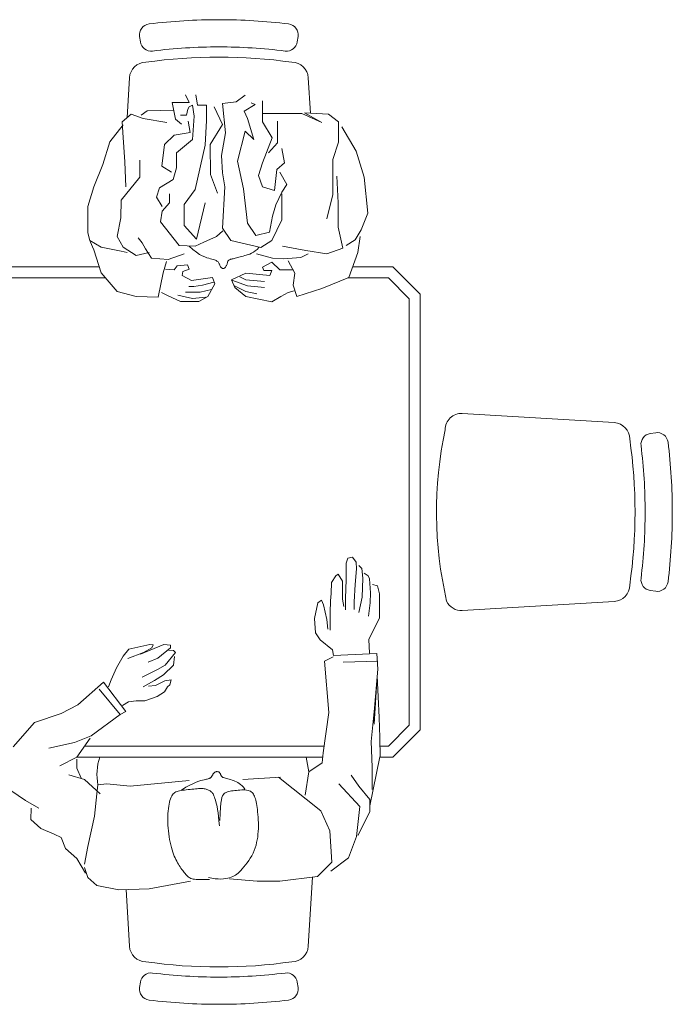
# Model space of a CAD drawing. Units: inches. Extents: x 1913 to 5309, y 1003 to 1733.
# Tile 6 of 23: x 2248 to 2284, y 1415 to 1469. Entities that reach past the tile are written whole.
import ezdxf

# ---------------------------------------------------------------- set-up
doc = ezdxf.new("R2010")
doc.units = ezdxf.units.IN
doc.layers.add('A-FURN', color=8, linetype='Continuous', lineweight=18)

# ---------------------------------------------------------------- blocks, each defined once
blk = doc.blocks.new('A$C421907B3')
for p, q in [((0.3742, 1.1891), (0.3928, 1.2157)), ((0.4726, 1.2115), (0.5176, 1.1724)), ((0.3229, 1.1605), (0.3394, 1.1788)), ((0.3394, 1.1788), (0.36, 1.1787)), ((0.36, 1.1646), (0.3742, 1.1891)), ((0.3126, 1.1359), (0.3229, 1.1605)), ((0.5176, 1.1724), (0.5341, 1.1234)), ((0.4808, 1.0989), (0.4706, 1.1459)), ((0.2861, 1.1152), (0.3066, 1.1235)), ((0.3066, 1.1235), (0.3126, 1.1359)), ((0.4378, 1.1255), (0.454, 1.0947)), ((0.5341, 1.1234), (0.5503, 1.0926)), ((0.2676, 1.0948), (0.2861, 1.1152)), ((0.4132, 1.0806), (0.4212, 1.1093)), ((0.241, 1.0786), (0.2676, 1.0948)), ((0.4335, 1.0947), (0.4152, 1.0865)), ((0.45, 1.0947), (0.4335, 1.0947)), ((0.454, 1.0947), (0.489, 1.0702)), ((0.493, 1.0681), (0.4808, 1.0989)), ((0.5503, 1.0926), (0.5914, 1.0456)), ((0.2328, 1.0745), (0.2183, 1.0579)), ((0.2511, 1.0807), (0.2328, 1.0745)), ((0.2573, 1.0807), (0.2901, 1.0744)), ((0.2901, 1.0744), (0.3454, 1.062)), ((0.3864, 1.0516), (0.4132, 1.0806)), ((0.5322, 1.015), (0.493, 1.0681)), ((1.3858, 1.0635), (1.4011, 1.0699)), ((1.4031, 1.0709), (1.3905, 1.0498)), ((1.4171, 1.0745), (1.4031, 1.0709)), ((1.4656, 1.0745), (1.4171, 1.0745)), ((1.5014, 1.0634), (1.4656, 1.0745)), ((0.2183, 1.0579), (0.2102, 1.0171)), ((0.3454, 1.062), (0.3864, 1.0578)), ((0.3864, 1.0578), (0.4029, 1.0557)), ((0.4029, 1.0557), (0.4049, 1.0395)), ((0.5791, 1.0535), (0.532, 1.0149)), ((1.3094, 1.0205), (1.3433, 1.0498)), ((1.3433, 1.0498), (1.3858, 1.0635)), ((1.3905, 1.0498), (1.3831, 1.0131)), ((1.5426, 1.0469), (1.5014, 1.0634)), ((0.4049, 1.0395), (0.4006, 0.9963)), ((0.538, 1.0045), (0.5914, 1.0456)), ((0.5958, 1.0315), (0.5832, 1.0366)), ((0.618, 1.0218), (0.5958, 1.0315)), ((1.5838, 1.034), (1.5426, 1.0469)), ((1.615, 1.0092), (1.5838, 1.034)), ((0.2102, 1.0171), (0.2122, 0.9615)), ((0.532, 1.0149), (0.538, 1.0045)), ((0.6395, 1.0092), (0.618, 1.0218)), ((1.3001, 0.9856), (1.3094, 1.0205)), ((1.3831, 1.0131), (1.3811, 1.0021)), ((1.3904, 1.0094), (1.4104, 1.0204)), ((1.4104, 1.0204), (1.4443, 1.0139)), ((1.4443, 1.0139), (1.4768, 1.013)), ((1.4768, 1.013), (1.5193, 0.979)), ((0.4006, 0.9963), (0.4108, 0.8878)), ((0.5491, 1.0108), (0.5557, 0.9996)), ((0.5557, 0.9996), (0.5572, 0.9855)), ((0.635, 1.001), (0.6461, 0.9722)), ((0.6521, 0.9988), (0.6395, 1.0092)), ((0.6609, 0.9603), (0.6521, 0.9988)), ((1.3751, 0.9856), (1.3904, 1.0094)), ((1.5014, 1.0047), (1.5472, 1.0065)), ((1.5472, 1.0065), (1.5918, 1.0092)), ((1.5918, 1.0092), (1.621, 1.011)), ((1.621, 1.011), (1.6349, 0.9945)), ((0.5572, 0.9855), (0.5572, 0.9693)), ((0.6609, 0.9344), (0.6432, 0.9774)), ((1.2987, 0.9453), (1.3001, 0.9856)), ((1.3811, 0.9617), (1.3751, 0.9856)), ((1.3984, 0.9745), (1.4077, 0.9819)), ((1.5193, 0.979), (1.5505, 0.979)), ((1.6349, 0.9945), (1.627, 0.9725)), ((0.2122, 0.9615), (0.2264, 0.8858)), ((0.5572, 0.9693), (0.5653, 0.947)), ((0.5832, 0.9729), (0.595, 0.9515)), ((0.5854, 0.9499), (0.5846, 0.9626)), ((0.6009, 0.9744), (0.615, 0.9462)), ((0.6283, 0.9633), (0.6357, 0.9455)), ((0.6461, 0.9722), (0.655, 0.9566)), ((0.6602, 0.9544), (0.6609, 0.9603)), ((1.3705, 0.9571), (1.3877, 0.9681)), ((1.3877, 0.9681), (1.3984, 0.9745)), ((1.627, 0.9725), (1.6196, 0.9294)), ((1.6409, 0.9652), (1.6329, 0.9762)), ((1.6421, 0.9163), (1.6409, 0.9652)), ((0.5653, 0.947), (0.5742, 0.9337)), ((0.5942, 0.933), (0.5854, 0.9499)), ((0.595, 0.9515), (0.6053, 0.9352)), ((0.615, 0.9462), (0.6232, 0.9322)), ((0.6357, 0.9455), (0.655, 0.9225)), ((0.655, 0.9566), (0.6602, 0.9544)), ((1.3432, 0.9361), (1.2987, 0.9453)), ((1.3678, 0.9269), (1.3705, 0.9571)), ((1.3937, 0.9067), (1.4369, 0.9406)), ((1.4369, 0.9406), (1.4568, 0.9378)), ((1.4655, 0.9378), (1.4827, 0.9479)), ((1.4827, 0.9479), (1.4994, 0.9423)), ((1.4994, 0.9423), (1.5146, 0.9176)), ((0.2929, 0.922), (0.2977, 0.923)), ((0.2977, 0.923), (0.3027, 0.924)), ((0.3027, 0.924), (0.3078, 0.9248)), ((0.3078, 0.9248), (0.3131, 0.9255)), ((0.3131, 0.9255), (0.3184, 0.9261)), ((0.3184, 0.9261), (0.3238, 0.9266)), ((0.3238, 0.9266), (0.3293, 0.927)), ((0.3293, 0.927), (0.3347, 0.9272)), ((0.3347, 0.9272), (0.34, 0.9272)), ((0.34, 0.9272), (0.3452, 0.9272)), ((0.3452, 0.9272), (0.3502, 0.927)), ((0.3502, 0.927), (0.355, 0.9267)), ((0.355, 0.9267), (0.3595, 0.9262)), ((0.3595, 0.9262), (0.3638, 0.9257)), ((0.3638, 0.9257), (0.3677, 0.925)), ((0.3677, 0.925), (0.3713, 0.9242)), ((0.3713, 0.9242), (0.3746, 0.9233)), ((0.3746, 0.9233), (0.3776, 0.9223)), ((0.3776, 0.9223), (0.3803, 0.9212)), ((0.5742, 0.9337), (0.5832, 0.9278)), ((0.5832, 0.9278), (0.5869, 0.9233)), ((0.5869, 0.9233), (0.5957, 0.9211)), ((0.5957, 0.9211), (0.5942, 0.933)), ((0.6053, 0.9352), (0.6232, 0.9166)), ((0.6232, 0.9322), (0.6461, 0.9129)), ((0.6498, 0.9166), (0.6506, 0.9263)), ((0.655, 0.9225), (0.6594, 0.9225)), ((0.6594, 0.9225), (0.6609, 0.9344)), ((1.2907, 0.904), (1.3013, 0.9269)), ((1.3013, 0.9269), (1.3073, 0.9388)), ((1.3645, 0.9296), (1.3432, 0.9361)), ((1.3505, 0.9315), (1.3492, 0.9159)), ((1.3784, 0.8975), (1.3678, 0.9269)), ((1.4568, 0.9378), (1.4721, 0.924)), ((1.4721, 0.924), (1.4887, 0.924)), ((1.5286, 0.9203), (1.5392, 0.9386)), ((1.5392, 0.9386), (1.5791, 0.9331)), ((1.5791, 0.9331), (1.5963, 0.9157)), ((0.25, 0.9031), (0.2524, 0.9047)), ((0.2524, 0.9047), (0.2548, 0.9063)), ((0.2548, 0.9063), (0.2573, 0.9078)), ((0.2573, 0.9078), (0.26, 0.9094)), ((0.26, 0.9094), (0.2628, 0.911)), ((0.2628, 0.911), (0.2657, 0.9125)), ((0.2657, 0.9125), (0.2689, 0.914)), ((0.2689, 0.914), (0.2723, 0.9155)), ((0.2723, 0.9155), (0.2759, 0.9169)), ((0.2759, 0.9169), (0.2797, 0.9183)), ((0.2797, 0.9183), (0.2839, 0.9196)), ((0.2839, 0.9196), (0.2883, 0.9208)), ((0.2883, 0.9208), (0.2929, 0.922)), ((0.3803, 0.9212), (0.3826, 0.92)), ((0.3826, 0.92), (0.3847, 0.9187)), ((0.3847, 0.9187), (0.3864, 0.9173)), ((0.3864, 0.9173), (0.3878, 0.9158)), ((0.3878, 0.9158), (0.389, 0.9142)), ((0.389, 0.9142), (0.39, 0.9123)), ((0.39, 0.9123), (0.3908, 0.9104)), ((0.3908, 0.9104), (0.3915, 0.9081)), ((0.3915, 0.9081), (0.3921, 0.9057)), ((0.3921, 0.9057), (0.3926, 0.903)), ((0.6232, 0.9166), (0.6387, 0.9151)), ((0.6461, 0.9129), (0.6498, 0.9166)), ((1.2965, 0.8821), (1.3022, 0.9091)), ((1.3492, 0.9159), (1.3565, 0.9104)), ((1.3565, 0.9104), (1.3584, 0.8911)), ((1.3923, 0.8773), (1.3937, 0.9067)), ((1.5146, 0.9176), (1.5365, 0.9111)), ((1.5365, 0.9111), (1.5638, 0.9111)), ((1.5638, 0.9111), (1.5883, 0.8817)), ((1.5963, 0.9157), (1.601, 0.8863)), ((1.6163, 0.9019), (1.6256, 0.9129)), ((1.6256, 0.9129), (1.6561, 0.9193)), ((1.6561, 0.9193), (1.6561, 0.8881)), ((0.2313, 0.8848), (0.2322, 0.8866)), ((0.2322, 0.8866), (0.2332, 0.8883)), ((0.2332, 0.8883), (0.2343, 0.8898)), ((0.2343, 0.8898), (0.2356, 0.8913)), ((0.2356, 0.8913), (0.237, 0.8927)), ((0.237, 0.8927), (0.2385, 0.8941)), ((0.2385, 0.8941), (0.2401, 0.8956)), ((0.2401, 0.8956), (0.2419, 0.897)), ((0.2419, 0.897), (0.2437, 0.8985)), ((0.2437, 0.8985), (0.2457, 0.9)), ((0.2457, 0.9), (0.2478, 0.9016)), ((0.2478, 0.9016), (0.25, 0.9031)), ((0.3926, 0.903), (0.3931, 0.8999)), ((0.3931, 0.8999), (0.3935, 0.8967)), ((0.3935, 0.8967), (0.394, 0.8933)), ((0.3936, 0.9023), (0.3986, 0.894)), ((0.394, 0.8933), (0.3944, 0.8898)), ((0.3944, 0.8898), (0.3947, 0.8863)), ((0.3947, 0.8863), (0.3951, 0.8829)), ((0.3986, 0.894), (0.4026, 0.8867)), ((0.4026, 0.8867), (0.4057, 0.8804)), ((1.2906, 0.87), (1.2907, 0.904)), ((1.3079, 0.8681), (1.3079, 0.8945)), ((1.3183, 0.8795), (1.3183, 0.8888)), ((1.3385, 0.9012), (1.3292, 0.8838)), ((1.3458, 0.8994), (1.3385, 0.9012)), ((1.3505, 0.8883), (1.3458, 0.8994)), ((1.3584, 0.8911), (1.3505, 0.8883)), ((1.3861, 0.8811), (1.3923, 0.8883)), ((1.4056, 0.8745), (1.4302, 0.8974)), ((1.4302, 0.8974), (1.4687, 0.8974)), ((1.4687, 0.8974), (1.4966, 0.8772)), ((1.601, 0.8863), (1.6222, 0.8899)), ((1.6329, 0.8927), (1.6329, 0.9037)), ((1.6442, 0.8908), (1.6329, 0.8927)), ((1.6481, 0.8881), (1.6442, 0.8908)), ((1.6515, 0.8817), (1.6481, 0.8881)), ((1.6561, 0.8881), (1.6701, 0.8945)), ((0.2291, 0.8687), (0.2292, 0.8722)), ((0.2291, 0.8649), (0.2291, 0.8687)), ((0.2292, 0.8722), (0.2294, 0.8753)), ((0.2294, 0.8753), (0.2297, 0.8781)), ((0.2297, 0.8781), (0.2301, 0.8806)), ((0.2301, 0.8806), (0.2306, 0.8828)), ((0.2306, 0.8828), (0.2313, 0.8848)), ((0.3951, 0.8829), (0.3954, 0.8796)), ((0.3954, 0.8796), (0.3957, 0.8765)), ((0.3957, 0.8765), (0.3959, 0.8736)), ((0.3959, 0.8736), (0.3961, 0.871)), ((0.3961, 0.871), (0.3962, 0.8685)), ((0.3962, 0.8685), (0.3962, 0.8663)), ((0.4057, 0.8804), (0.4081, 0.8751)), ((0.4081, 0.8751), (0.4098, 0.8705)), ((0.4098, 0.8705), (0.411, 0.8667)), ((1.2999, 0.8535), (1.2906, 0.87)), ((1.2985, 0.8577), (1.2965, 0.8821)), ((1.3126, 0.8473), (1.3079, 0.8681)), ((1.3209, 0.8634), (1.3183, 0.8795)), ((1.3292, 0.8838), (1.3351, 0.8452)), ((1.3746, 0.864), (1.3774, 0.869)), ((1.3774, 0.869), (1.3812, 0.8747)), ((1.3812, 0.8747), (1.3861, 0.8811)), ((1.3996, 0.8608), (1.3923, 0.8773)), ((1.472, 0.8589), (1.4056, 0.8745)), ((1.4966, 0.8772), (1.5777, 0.8588)), ((1.5883, 0.8817), (1.6315, 0.8789)), ((1.6315, 0.8789), (1.6515, 0.8817)), ((1.6514, 0.8725), (1.6701, 0.8761)), ((1.6514, 0.856), (1.6514, 0.8725)), ((0.2291, 0.8607), (0.2291, 0.8649)), ((0.2291, 0.856), (0.2291, 0.8607)), ((0.2291, 0.8509), (0.2291, 0.856)), ((0.2316, 0.8463), (0.2331, 0.8527)), ((0.3927, 0.8508), (0.3918, 0.8495)), ((0.3934, 0.8523), (0.3927, 0.8508)), ((0.3941, 0.8538), (0.3934, 0.8523)), ((0.3947, 0.8553), (0.3941, 0.8538)), ((0.3952, 0.857), (0.3947, 0.8553)), ((0.3956, 0.8587), (0.3952, 0.857)), ((0.3959, 0.8604), (0.3956, 0.8587)), ((0.3961, 0.8623), (0.3959, 0.8604)), ((0.3962, 0.8642), (0.3961, 0.8623)), ((0.3962, 0.8663), (0.3962, 0.8642)), ((0.411, 0.8667), (0.4118, 0.8634)), ((0.4118, 0.8634), (0.4124, 0.8607)), ((0.4124, 0.8607), (0.4129, 0.8583)), ((0.4129, 0.8583), (0.4134, 0.8564)), ((0.4134, 0.8564), (0.4138, 0.8547)), ((0.4138, 0.8547), (0.4141, 0.8533)), ((0.4141, 0.8533), (0.4145, 0.8522)), ((0.4145, 0.8522), (0.4148, 0.8512)), ((0.4148, 0.8512), (0.4152, 0.8504)), ((0.4152, 0.8504), (0.4156, 0.8497)), ((1.3232, 0.8407), (1.2999, 0.8535)), ((1.3261, 0.8427), (1.3209, 0.8634)), ((1.3694, 0.849), (1.3702, 0.852)), ((1.3702, 0.852), (1.3712, 0.8555)), ((1.3712, 0.8555), (1.3726, 0.8595)), ((1.3726, 0.8595), (1.3746, 0.864)), ((1.4102, 0.8378), (1.3996, 0.8608)), ((1.5777, 0.8588), (1.6235, 0.856)), ((1.6235, 0.856), (1.6514, 0.856)), ((0.2301, 0.8299), (0.2302, 0.8349)), ((0.2302, 0.8349), (0.2307, 0.8404)), ((0.2307, 0.8404), (0.2316, 0.8463)), ((0.3369, 0.8333), (0.328, 0.8326)), ((0.3448, 0.8341), (0.3369, 0.8333)), ((0.3375, 0.8319), (0.3508, 0.8313)), ((0.3518, 0.835), (0.3448, 0.8341)), ((0.3579, 0.8359), (0.3518, 0.835)), ((0.3632, 0.8369), (0.3579, 0.8359)), ((0.3678, 0.8379), (0.3632, 0.8369)), ((0.3718, 0.8389), (0.3678, 0.8379)), ((0.3752, 0.8398), (0.3718, 0.8389)), ((0.3782, 0.8407), (0.3752, 0.8398)), ((0.3807, 0.8416), (0.3782, 0.8407)), ((0.3829, 0.8425), (0.3807, 0.8416)), ((0.3847, 0.8433), (0.3829, 0.8425)), ((0.3863, 0.8442), (0.3847, 0.8433)), ((0.3876, 0.8451), (0.3863, 0.8442)), ((0.3888, 0.846), (0.3876, 0.8451)), ((0.3899, 0.8471), (0.3888, 0.846)), ((0.3909, 0.8482), (0.3899, 0.8471)), ((0.3918, 0.8495), (0.3909, 0.8482)), ((0.4156, 0.8497), (0.416, 0.849)), ((0.416, 0.849), (0.4165, 0.8484)), ((0.4165, 0.8484), (0.417, 0.8478)), ((0.417, 0.8478), (0.4176, 0.8473)), ((0.4176, 0.8473), (0.4182, 0.8468)), ((0.4182, 0.8468), (0.4188, 0.8463)), ((0.4188, 0.8463), (0.4195, 0.8459)), ((0.4195, 0.8459), (0.4202, 0.8455)), ((0.4202, 0.8455), (0.4209, 0.8451)), ((0.4209, 0.8451), (0.4217, 0.8448)), ((0.4217, 0.8448), (0.4225, 0.8444)), ((0.4225, 0.8444), (0.4233, 0.8439)), ((0.4233, 0.8439), (0.424, 0.8435)), ((0.424, 0.8435), (0.4247, 0.8429)), ((0.4247, 0.8429), (0.4253, 0.8423)), ((0.4255, 0.8322), (0.4248, 0.8316)), ((0.4253, 0.8423), (0.4259, 0.8415)), ((0.4261, 0.8329), (0.4255, 0.8322)), ((0.4259, 0.8415), (0.4264, 0.8407)), ((0.4267, 0.8337), (0.4261, 0.8329)), ((0.4264, 0.8407), (0.4268, 0.8397)), ((0.427, 0.8346), (0.4267, 0.8337)), ((0.4268, 0.8397), (0.4271, 0.8387)), ((0.4272, 0.8356), (0.427, 0.8346)), ((0.4271, 0.8387), (0.4273, 0.8377)), ((0.4273, 0.8366), (0.4272, 0.8356)), ((0.4273, 0.8377), (0.4273, 0.8366)), ((1.3351, 0.8452), (1.3232, 0.8407)), ((1.3568, 0.8316), (1.3579, 0.832)), ((1.3579, 0.832), (1.3591, 0.8325)), ((1.3591, 0.8325), (1.3602, 0.833)), ((1.3602, 0.833), (1.3613, 0.8335)), ((1.3613, 0.8335), (1.3624, 0.8342)), ((1.3624, 0.8342), (1.3634, 0.835)), ((1.3634, 0.835), (1.3643, 0.8359)), ((1.3643, 0.8359), (1.3651, 0.837)), ((1.3651, 0.837), (1.3659, 0.8384)), ((1.3659, 0.8384), (1.3666, 0.8399)), ((1.3666, 0.8399), (1.3673, 0.8417)), ((1.3673, 0.8417), (1.368, 0.8438)), ((1.368, 0.8438), (1.3687, 0.8462)), ((1.3687, 0.8462), (1.3694, 0.849)), ((1.4208, 0.8259), (1.4102, 0.8378)), ((1.49, 0.8359), (1.5239, 0.8487)), ((1.5239, 0.8487), (1.579, 0.8496)), ((1.579, 0.8496), (1.6162, 0.8266)), ((1.6162, 0.8266), (1.6481, 0.8422)), ((0.2306, 0.814), (0.2263, 0.7628)), ((0.2304, 0.8252), (0.2301, 0.8299)), ((0.2309, 0.821), (0.2304, 0.8252)), ((0.2316, 0.8172), (0.2309, 0.821)), ((0.2325, 0.8138), (0.2316, 0.8172)), ((0.3508, 0.8313), (0.3614, 0.8306)), ((0.3614, 0.8306), (0.3695, 0.8298)), ((0.3695, 0.8298), (0.3757, 0.8289)), ((0.3757, 0.8289), (0.3801, 0.8278)), ((0.3801, 0.8278), (0.3832, 0.8265)), ((0.3832, 0.8265), (0.3854, 0.8251)), ((0.3854, 0.8251), (0.3869, 0.8235)), ((0.3869, 0.8235), (0.3882, 0.8218)), ((0.3882, 0.8218), (0.3892, 0.8198)), ((0.3892, 0.8198), (0.3901, 0.8176)), ((0.3901, 0.8176), (0.3908, 0.8153)), ((0.3908, 0.8153), (0.3914, 0.8128)), ((0.4133, 0.8145), (0.4126, 0.8119)), ((0.414, 0.8169), (0.4133, 0.8145)), ((0.4147, 0.8192), (0.414, 0.8169)), ((0.4152, 0.8213), (0.4147, 0.8192)), ((0.4158, 0.8231), (0.4152, 0.8213)), ((0.4163, 0.8247), (0.4158, 0.8231)), ((0.4168, 0.826), (0.4163, 0.8247)), ((0.4173, 0.827), (0.4168, 0.826)), ((0.4178, 0.8277), (0.4173, 0.827)), ((0.4183, 0.8283), (0.4178, 0.8277)), ((0.4188, 0.8288), (0.4183, 0.8283)), ((0.4194, 0.8291), (0.4188, 0.8288)), ((0.42, 0.8294), (0.4194, 0.8291)), ((0.4207, 0.8297), (0.42, 0.8294)), ((0.4215, 0.83), (0.4207, 0.8297)), ((0.4223, 0.8303), (0.4215, 0.83)), ((0.4231, 0.8307), (0.4223, 0.8303)), ((0.424, 0.8311), (0.4231, 0.8307)), ((0.4248, 0.8316), (0.424, 0.8311)), ((1.3512, 0.826), (1.3514, 0.8269)), ((1.3512, 0.8251), (1.3512, 0.826)), ((1.3514, 0.8243), (1.3512, 0.8251)), ((1.3514, 0.8269), (1.3518, 0.8277)), ((1.3518, 0.8234), (1.3514, 0.8243)), ((1.3518, 0.8277), (1.3524, 0.8285)), ((1.3524, 0.8226), (1.3518, 0.8234)), ((1.3524, 0.8285), (1.353, 0.8292)), ((1.3531, 0.8218), (1.3524, 0.8226)), ((1.353, 0.8292), (1.3538, 0.8299)), ((1.354, 0.8211), (1.3531, 0.8218)), ((1.3538, 0.8299), (1.3547, 0.8305)), ((1.355, 0.8204), (1.354, 0.8211)), ((1.3547, 0.8305), (1.3557, 0.8311)), ((1.3561, 0.8198), (1.355, 0.8204)), ((1.3557, 0.8311), (1.3568, 0.8316)), ((1.3572, 0.8192), (1.3561, 0.8198)), ((1.3584, 0.8188), (1.3572, 0.8192)), ((1.3595, 0.8184), (1.3584, 0.8188)), ((1.3607, 0.8181), (1.3595, 0.8184)), ((1.3618, 0.8179), (1.3607, 0.8181)), ((1.3629, 0.8176), (1.3618, 0.8179)), ((1.3639, 0.8173), (1.3629, 0.8176)), ((1.3648, 0.8169), (1.3639, 0.8173)), ((1.3656, 0.8165), (1.3648, 0.8169)), ((1.3664, 0.8159), (1.3656, 0.8165)), ((1.367, 0.8151), (1.3664, 0.8159)), ((1.3675, 0.8141), (1.367, 0.8151)), ((1.3679, 0.813), (1.3675, 0.8141)), ((1.4029, 0.8112), (1.4255, 0.8268)), ((1.4255, 0.8268), (1.5012, 0.8222)), ((1.5012, 0.8222), (1.5272, 0.8267)), ((1.5272, 0.8267), (1.5591, 0.8285)), ((1.5591, 0.8285), (1.6009, 0.8212)), ((1.6009, 0.8212), (1.6547, 0.8266)), ((1.6547, 0.8266), (1.6574, 0.8018)), ((0.2335, 0.8107), (0.2325, 0.8138)), ((0.2346, 0.8079), (0.2335, 0.8107)), ((0.2359, 0.8053), (0.2346, 0.8079)), ((0.2374, 0.8029), (0.2359, 0.8053)), ((0.2391, 0.8006), (0.2374, 0.8029)), ((0.241, 0.7983), (0.2391, 0.8006)), ((0.2433, 0.7958), (0.241, 0.7983)), ((0.246, 0.7933), (0.2433, 0.7958)), ((0.3914, 0.8128), (0.3919, 0.8101)), ((0.3919, 0.8101), (0.3923, 0.8073)), ((0.3923, 0.8073), (0.3926, 0.8043)), ((0.3926, 0.8043), (0.393, 0.8012)), ((0.393, 0.8012), (0.3933, 0.7979)), ((0.3933, 0.7979), (0.3936, 0.7947)), ((0.4057, 0.796), (0.4037, 0.7935)), ((0.4073, 0.7987), (0.4057, 0.796)), ((0.4087, 0.8013), (0.4073, 0.7987)), ((0.4098, 0.804), (0.4087, 0.8013)), ((0.4108, 0.8066), (0.4098, 0.804)), ((0.4117, 0.8093), (0.4108, 0.8066)), ((0.4126, 0.8119), (0.4117, 0.8093)), ((1.2999, 0.7838), (1.3165, 0.804)), ((1.3089, 0.784), (1.3203, 0.8058)), ((1.3165, 0.804), (1.3305, 0.8104)), ((1.3193, 0.7809), (1.3297, 0.8099)), ((1.3305, 0.8104), (1.3431, 0.7838)), ((1.3683, 0.8118), (1.3679, 0.813)), ((1.3686, 0.8104), (1.3683, 0.8118)), ((1.369, 0.8088), (1.3686, 0.8104)), ((1.3694, 0.8071), (1.369, 0.8088)), ((1.3698, 0.8053), (1.3694, 0.8071)), ((1.3703, 0.8033), (1.3698, 0.8053)), ((1.3708, 0.8013), (1.3703, 0.8033)), ((1.3714, 0.799), (1.3708, 0.8013)), ((1.3721, 0.7967), (1.3714, 0.799)), ((1.3728, 0.7942), (1.3721, 0.7967)), ((1.3902, 0.7562), (1.4029, 0.8112)), ((1.4979, 0.7882), (1.5484, 0.7992)), ((1.5484, 0.7992), (1.6035, 0.7854)), ((1.6574, 0.8018), (1.67, 0.7853)), ((0.249, 0.7905), (0.246, 0.7933)), ((0.2523, 0.7876), (0.249, 0.7905)), ((0.256, 0.7846), (0.2523, 0.7876)), ((0.2599, 0.7816), (0.256, 0.7846)), ((0.264, 0.7786), (0.2599, 0.7816)), ((0.2684, 0.7758), (0.264, 0.7786)), ((0.3923, 0.7776), (0.3914, 0.7756)), ((0.393, 0.7799), (0.3923, 0.7776)), ((0.3934, 0.7825), (0.393, 0.7799)), ((0.3937, 0.7853), (0.3934, 0.7825)), ((0.3936, 0.7947), (0.3937, 0.7915)), ((0.3937, 0.7915), (0.3938, 0.7883)), ((0.3938, 0.7883), (0.3937, 0.7853)), ((0.3986, 0.7884), (0.3953, 0.7859)), ((0.4014, 0.7909), (0.3986, 0.7884)), ((0.4037, 0.7935), (0.4014, 0.7909)), ((0.413, 0.7893), (0.417, 0.7199)), ((1.2905, 0.7361), (1.2999, 0.7838)), ((1.3047, 0.7638), (1.3089, 0.784)), ((1.3166, 0.7498), (1.3193, 0.7809)), ((1.3275, 0.7498), (1.3307, 0.784)), ((1.3307, 0.784), (1.3359, 0.7949)), ((1.3431, 0.7838), (1.3384, 0.7397)), ((1.3736, 0.7916), (1.3728, 0.7942)), ((1.3743, 0.7889), (1.3736, 0.7916)), ((1.3751, 0.786), (1.3743, 0.7889)), ((1.376, 0.783), (1.3751, 0.786)), ((1.3769, 0.7799), (1.376, 0.783)), ((1.378, 0.7767), (1.3769, 0.7799)), ((1.4122, 0.7654), (1.4348, 0.7809)), ((1.4348, 0.7809), (1.4979, 0.7882)), ((1.6035, 0.7854), (1.5882, 0.7689)), ((1.5882, 0.7689), (1.6268, 0.7808)), ((1.6268, 0.7808), (1.6407, 0.7872)), ((1.6407, 0.7872), (1.6527, 0.767)), ((0.2263, 0.7628), (0.2263, 0.7217)), ((0.2729, 0.7731), (0.2684, 0.7758)), ((0.2776, 0.7707), (0.2729, 0.7731)), ((0.2823, 0.7686), (0.2776, 0.7707)), ((0.2871, 0.7668), (0.2823, 0.7686)), ((0.292, 0.7652), (0.2871, 0.7668)), ((0.297, 0.764), (0.292, 0.7652)), ((0.302, 0.7629), (0.297, 0.764)), ((0.3071, 0.7621), (0.302, 0.7629)), ((0.3123, 0.7616), (0.3071, 0.7621)), ((0.3176, 0.7612), (0.3123, 0.7616)), ((0.3229, 0.7609), (0.3176, 0.7612)), ((0.3282, 0.7609), (0.3229, 0.7609)), ((0.3335, 0.7609), (0.3282, 0.7609)), ((0.3387, 0.7611), (0.3335, 0.7609)), ((0.3438, 0.7614), (0.3387, 0.7611)), ((0.3486, 0.7618), (0.3438, 0.7614)), ((0.3533, 0.7622), (0.3486, 0.7618)), ((0.3576, 0.7627), (0.3533, 0.7622)), ((0.3617, 0.7632), (0.3576, 0.7627)), ((0.3654, 0.7637), (0.3617, 0.7632)), ((0.3688, 0.7643), (0.3654, 0.7637)), ((0.3719, 0.7649), (0.3688, 0.7643)), ((0.3748, 0.7656), (0.3719, 0.7649)), ((0.3774, 0.7663), (0.3748, 0.7656)), ((0.3799, 0.7671), (0.3774, 0.7663)), ((0.3821, 0.768), (0.3799, 0.7671)), ((0.3841, 0.7689), (0.3821, 0.768)), ((0.386, 0.7699), (0.3841, 0.7689)), ((0.3876, 0.7711), (0.386, 0.7699)), ((0.3891, 0.7724), (0.3876, 0.7711)), ((0.3904, 0.7739), (0.3891, 0.7724)), ((0.3914, 0.7756), (0.3904, 0.7739)), ((1.3703, 0.7351), (1.3783, 0.7645)), ((1.3795, 0.7735), (1.378, 0.7767)), ((1.3813, 0.7701), (1.3795, 0.7735)), ((1.3837, 0.7667), (1.3813, 0.7701)), ((1.3866, 0.7633), (1.3837, 0.7667)), ((1.3902, 0.7599), (1.3866, 0.7633)), ((1.4181, 0.7406), (1.4122, 0.7654)), ((1.5012, 0.7534), (1.5224, 0.7607)), ((1.5224, 0.7607), (1.5457, 0.7533)), ((1.6527, 0.767), (1.656, 0.7743)), ((1.3477, 0.7507), (1.3537, 0.7535)), ((1.3477, 0.7361), (1.3477, 0.7507)), ((1.3537, 0.7535), (1.363, 0.736)), ((1.4028, 0.736), (1.3902, 0.7562)), ((1.4945, 0.7313), (1.5012, 0.7534)), ((1.5457, 0.7533), (1.5915, 0.7358)), ((1.5822, 0.7258), (1.5636, 0.7423)), ((1.5915, 0.7358), (1.6208, 0.7532)), ((1.6208, 0.7532), (1.6593, 0.7532)), ((1.6361, 0.7532), (1.636, 0.6808)), ((0.3554, 0.646), (0.417, 0.7237)), ((1.2998, 0.7196), (1.2905, 0.7361)), ((1.3384, 0.7397), (1.3477, 0.7361)), ((1.363, 0.736), (1.349, 0.7214)), ((1.3689, 0.7149), (1.3703, 0.7351)), ((1.4407, 0.7176), (1.4028, 0.736)), ((1.4473, 0.7351), (1.4181, 0.7406)), ((1.4686, 0.7286), (1.4473, 0.7351)), ((1.4918, 0.7176), (1.4686, 0.7286)), ((1.5331, 0.7267), (1.4945, 0.7313)), ((1.5457, 0.7129), (1.5331, 0.7267)), ((1.6221, 0.7257), (1.5822, 0.7258)), ((0.2263, 0.7217), (0.2345, 0.6523)), ((1.3071, 0.7058), (1.2998, 0.7196)), ((1.3104, 0.6948), (1.3071, 0.7058)), ((1.343, 0.6939), (1.3656, 0.7058)), ((1.349, 0.7214), (1.349, 0.6984)), ((1.3716, 0.6828), (1.3689, 0.7149)), ((1.3842, 0.6736), (1.3922, 0.7167)), ((1.4885, 0.7176), (1.4407, 0.7176)), ((1.5058, 0.7084), (1.4918, 0.7176)), ((1.5284, 0.7212), (1.5058, 0.7084)), ((1.5716, 0.7175), (1.5457, 0.7129)), ((1.2998, 0.6902), (1.3211, 0.6966)), ((1.315, 0.6443), (1.2998, 0.6902)), ((1.3211, 0.6966), (1.343, 0.6939)), ((0.3842, 0.6746), (0.4272, 0.6684)), ((0.4272, 0.6684), (0.4542, 0.6729)), ((1.3782, 0.6691), (1.3716, 0.6828)), ((1.3782, 0.6351), (1.3842, 0.6736)), ((1.636, 0.6808), (1.6194, 0.6441)), ((1.6194, 0.6441), (1.6373, 0.6762)), ((1.6373, 0.6762), (1.6346, 0.6321)), ((0.2345, 0.6523), (0.261, 0.6256)), ((0.4272, 0.6684), (0.4435, 0.6438)), ((0.6692, 0.647), (0.6821, 0.6561)), ((0.6821, 0.6561), (0.7085, 0.6576)), ((0.7085, 0.6576), (0.7372, 0.6515)), ((0.7372, 0.6515), (0.7425, 0.6447)), ((0.3186, 0.6294), (0.3554, 0.646)), ((0.4435, 0.6438), (0.462, 0.6418)), ((0.462, 0.6418), (0.5358, 0.6313)), ((0.5358, 0.6313), (0.6302, 0.6396)), ((0.6302, 0.6396), (0.6381, 0.6233)), ((0.6511, 0.6244), (0.6692, 0.647)), ((0.707, 0.6349), (0.6889, 0.6334)), ((0.7335, 0.6409), (0.707, 0.6349)), ((0.7425, 0.6447), (0.7335, 0.6409)), ((1.3349, 0.5948), (1.315, 0.6443)), ((1.3888, 0.6057), (1.3782, 0.6351)), ((1.4871, 0.624), (1.4426, 0.6351)), ((0.2448, 0.6277), (0.2693, 0.5949)), ((0.261, 0.6256), (0.3186, 0.6294)), ((0.6405, 0.6229), (0.6511, 0.6244)), ((0.6405, 0.6229), (0.6444, 0.5432)), ((0.6873, 0.6288), (0.7199, 0.6288)), ((0.7199, 0.6288), (0.741, 0.6281)), ((0.741, 0.6281), (0.7546, 0.6273)), ((0.7546, 0.6273), (0.775, 0.6265)), ((0.775, 0.6265), (0.787, 0.6183)), ((0.787, 0.6183), (0.7901, 0.6144)), ((1.521, 0.6166), (1.4718, 0.6139)), ((1.5516, 0.624), (1.4871, 0.624)), ((1.5835, 0.6138), (1.5516, 0.624)), ((1.6346, 0.6321), (1.6207, 0.6138)), ((0.3636, 0.5741), (0.4047, 0.6131)), ((0.6281, 0.6047), (0.6301, 0.5411)), ((0.7243, 0.6009), (0.7462, 0.6009)), ((0.744, 0.6062), (0.7304, 0.6039)), ((0.7621, 0.6062), (0.744, 0.6062)), ((0.7462, 0.6009), (0.7795, 0.5993)), ((0.7772, 0.6062), (0.7621, 0.6062)), ((0.7901, 0.6144), (0.7772, 0.6062)), ((0.7795, 0.5993), (0.8105, 0.5993)), ((0.8105, 0.5993), (0.8195, 0.5963)), ((1.4273, 0.614), (1.3888, 0.6057)), ((1.404, 0.5828), (1.3934, 0.5993)), ((1.4718, 0.6139), (1.4273, 0.614)), ((1.6114, 0.6074), (1.5668, 0.5808)), ((1.6207, 0.6138), (1.5835, 0.6138)), ((0.2693, 0.5949), (0.3083, 0.5804)), ((0.3083, 0.5804), (0.3636, 0.5741)), ((0.4004, 0.5761), (0.4209, 0.5906)), ((0.7395, 0.585), (0.7251, 0.585)), ((0.7712, 0.5828), (0.7395, 0.585)), ((0.7999, 0.5804), (0.7712, 0.5828)), ((0.8119, 0.5812), (0.7999, 0.5804)), ((0.8211, 0.588), (0.8119, 0.5812)), ((0.8195, 0.5963), (0.8211, 0.588)), ((1.3808, 0.5782), (1.3349, 0.5948)), ((1.4226, 0.5718), (1.404, 0.5828)), ((1.5668, 0.5808), (1.519, 0.5662)), ((0.3103, 0.5783), (0.3533, 0.5558)), ((0.3759, 0.5558), (0.4004, 0.5761)), ((0.7198, 0.576), (0.7477, 0.5699)), ((0.7477, 0.5699), (0.7825, 0.5691)), ((0.7825, 0.5691), (0.8006, 0.5707)), ((0.787, 0.5593), (0.7916, 0.5661)), ((0.8006, 0.5707), (0.8059, 0.576)), ((1.41, 0.5736), (1.3808, 0.5782)), ((1.4532, 0.5598), (1.4226, 0.5718)), ((1.519, 0.5662), (1.4532, 0.5598)), ((0.3533, 0.5558), (0.3759, 0.5558)), ((0.4543, 0.5377), (0.3646, 0.5558)), ((0.4354, 0.5516), (0.3944, 0.5516)), ((0.4825, 0.5536), (0.4354, 0.5516)), ((0.544, 0.5474), (0.4825, 0.5536)), ((0.6156, 0.5411), (0.544, 0.5474)), ((0.6444, 0.5432), (0.6156, 0.5411)), ((0.645, 0.5564), (0.6699, 0.5579)), ((0.6699, 0.5579), (0.6926, 0.5466)), ((0.6926, 0.5466), (0.7092, 0.5382)), ((0.713, 0.5586), (0.7372, 0.5555)), ((0.7372, 0.5555), (0.756, 0.5548)), ((0.756, 0.5548), (0.7817, 0.5563)), ((0.7689, 0.5419), (0.7711, 0.551)), ((0.7817, 0.5563), (0.787, 0.5593)), ((0.7092, 0.5382), (0.7538, 0.5382)), ((0.7538, 0.5382), (0.7689, 0.5419))]:
    blk.add_line(p, q)
at = {"ltscale": 0.1}
for points in [[(1.2446, 2.3436), (1.3042, 2.3436), (1.3542, 2.2936), (1.3542, 1.0533)], [(1.245, 2.3234), (1.2959, 2.3236), (1.3342, 2.2853), (1.3342, 1.0419)], [(0.4542, 0.6426), (0.4542, 1.0946)], [(0.4742, 0.64), (0.4742, 1.0806)], [(1.3542, 0.5878), (1.3542, 0.5135), (1.3042, 0.4635), (0.5042, 0.4635), (0.4542, 0.5135), (0.4542, 0.5377)], [(1.3342, 0.5966), (1.3342, 0.5218), (1.2959, 0.4835), (0.5125, 0.4835), (0.4742, 0.5218), (0.4742, 0.5375)]]:
    blk.add_lwpolyline(points, dxfattribs=at)
for points in [[(0.2107, 1.004), (0.1067, 0.9977, 0.399285), (0.0782, 0.9677, 0.071734), (0.0782, 0.6992, 0.399285), (0.1067, 0.6693), (0.2334, 0.6616)], [(1.6285, 1.0021), (1.7017, 0.9977, -0.399285), (1.7302, 0.9677, -0.071734), (1.7302, 0.6992, -0.399285), (1.7017, 0.6693), (1.6367, 0.6653)]]:
    blk.add_lwpolyline(points, format="xyb", dxfattribs=at)
for points in [[(0.05, 0.8335, -0.030867), (0.0575, 0.9554, 0.408428), (0.0405, 0.9777), (0.0306, 0.9791, 0.419966), (0.0079, 0.9618, 0.030916), (0, 0.8335, 0.030916), (0.0079, 0.7052, 0.419966), (0.0306, 0.6878), (0.0405, 0.6893, 0.408428), (0.0575, 0.7115, -0.030867)], [(1.7584, 0.8335, 0.030867), (1.7509, 0.9554, -0.408428), (1.7679, 0.9777), (1.7778, 0.9791, -0.419966), (1.8005, 0.9618, -0.030916), (1.8084, 0.8335, -0.030916), (1.8005, 0.7052, -0.419966), (1.7778, 0.6878), (1.7679, 0.6893, -0.408428), (1.7509, 0.7115, 0.030867)], [(0.77, 0.0782, -0.399285), (0.74, 0.1067), (0.7231, 0.3861, -0.305593), (0.7404, 0.4148, -0.109362), (1.0554, 0.4176, -0.429301), (1.0853, 0.3861), (1.0684, 0.1067, -0.399285), (1.0384, 0.0782, -0.071734)], [(0.9042, 0.05, 0.030867), (1.0261, 0.0575, -0.408428), (1.0484, 0.0405), (1.0498, 0.0306, -0.419966), (1.0325, 0.0079, -0.030916), (0.9042, 0, -0.030916), (0.7759, 0.0079, -0.419966), (0.7586, 0.0306), (0.76, 0.0405, -0.408428), (0.7823, 0.0575, 0.030867)]]:
    blk.add_lwpolyline(points, format="xyb", close=True, dxfattribs=at)
blk.add_lwpolyline([(0.5267, 0.5491), (0.5148, 0.5482), (0.6033, 0.5427), (0.6033, 0.5427), (0.5647, 0.5405), (0.5267, 0.5387), (0.4898, 0.5376), (0.4542, 0.5371)])
blk.add_arc((0.4222, 0.9527), 0.1048, 72.2191, 100.5893)

msp = doc.modelspace()

# ---------------------------------------------------------------- block references
at = {"layer": 'A-FURN', "xscale": 30.26057373645948, "yscale": 30.26057373645948, "zscale": 30.26057373645948, "rotation": 89.99999999999996}
msp.add_blockref('A$C421907B3', (2284.376, 1414.678), dxfattribs=at)

doc.saveas('drawing.dxf')
